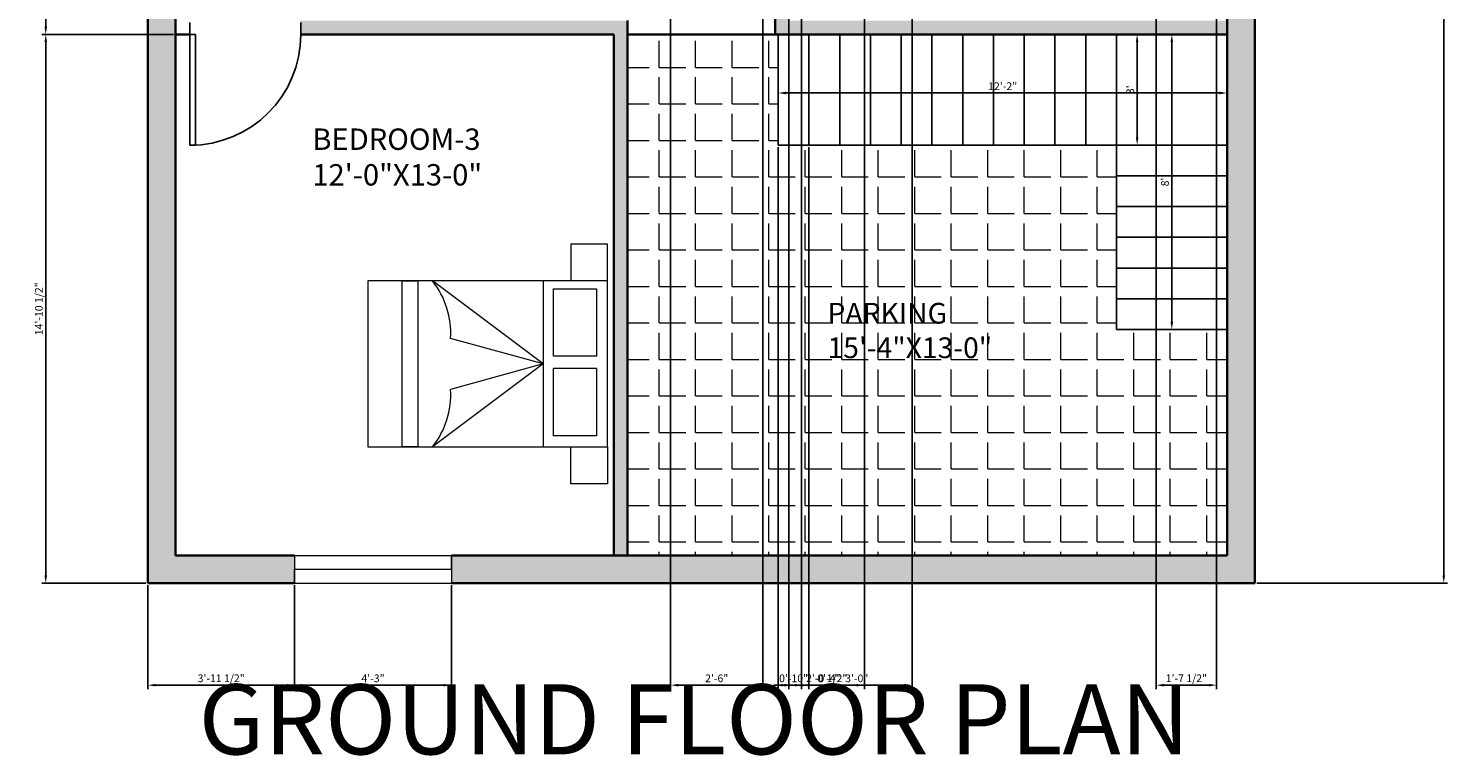
# Model space of a CAD drawing. Units: inches. Extents: x 2063 to 2524, y 2436 to 3097.
# Tile 1 of 4: x 2063 to 2524, y 2436 to 2673. Entities that reach past the tile are written whole.
import ezdxf

# ---------------------------------------------------------------- set-up
doc = ezdxf.new("R2010")
doc.units = ezdxf.units.IN
for name, color, linetype, lineweight in [('A-ANNO-DIMS', 2, 'Continuous', 18), ('A-ANNO-TEXT', 7, 'Continuous', 25), ('A-AREA-IDEN', 7, 'Continuous', 18), ('A-DOOR', 4, 'Continuous', 25), ('A-FLOR-STRS', 7, 'Continuous', 25), ('A-FURN', 8, 'Continuous', 18), ('A-GLAZ', 5, 'Continuous', 18), ('A-WALL', 7, 'Continuous', 35)]:
    doc.layers.add(name, color=color, linetype=linetype, lineweight=lineweight)
doc.layers.add('A-FLOR-PATT', color=252, linetype='Continuous', lineweight=13, true_color=0x939598)
doc.layers.add('A-WALL-PATT', color=251, linetype='Continuous', lineweight=13, true_color=0x636466)
doc.styles.get("Standard").update_dxf_attribs({"font": 'arial.ttf'})
doc.dimstyles.new('ISO-25', dxfattribs={"dimtxt": 2.5, "dimasz": 2.5, "dimexe": 1.25, "dimexo": 0.625, "dimtad": 1, "dimlunit": 3, "dimtxsty": 'Standard', "dimcen": 2.5, "dimadec": 0, "dimazin": 0, "dimtfac": 1, "dimtmove": 0, "dimatfit": 3, "dimfxl": 1, "dimarcsym": 0})

# ---------------------------------------------------------------- blocks, each defined once
blk = doc.blocks.new('*U7')
for p, q in [((0, 0), (0, 4)), ((36, 0), (36, 4))]:
    blk.add_line(p, q)
blk.add_lwpolyline([(0, 0), (0, -36), (1.75, -36), (1.75, 0)], close=True)
blk.add_arc((0, 0), 36, 270, 0)
blk = doc.blocks.new('*D8')
at = {"layer": 'A-ANNO-DIMS', "color": 0, "lineweight": -2, "transparency": 16777216}
for p, q in [((2306.76, 2669.99), (2306.76, 2650.32)), ((2452.76, 2669.99), (2452.76, 2650.32)), ((2450.26, 2651.57), (2309.26, 2651.57))]:
    blk.add_line(p, q, dxfattribs=at)
at = {"layer": 'A-ANNO-DIMS', "color": 0, "transparency": 16777216}
for points in [[(2309.26, 2651.99), (2309.26, 2651.15), (2306.76, 2651.57)], [(2450.26, 2651.99), (2450.26, 2651.15), (2452.76, 2651.57)]]:
    blk.add_solid(points, dxfattribs=at)
at = {"layer": 'Defpoints', "color": 0, "transparency": 16777216}
for p in [(2306.76, 2670.62), (2452.76, 2670.62), (2306.76, 2651.57)]:
    blk.add_point(p, dxfattribs=at)
at = {"layer": 'A-ANNO-DIMS', "color": 0, "transparency": 16777216, "insert": (2379.76, 2653.45), "char_height": 2.5, "attachment_point": 5}
blk.add_mtext('12\'-2"', dxfattribs=at)
blk = doc.blocks.new('*D9')
at = {"layer": 'A-ANNO-DIMS', "color": 0, "lineweight": -2, "transparency": 16777216}
for p, q in [((2452.14, 2670.62), (2433.51, 2670.62)), ((2434.76, 2668.12), (2434.76, 2577.12)), ((2452.14, 2574.62), (2433.51, 2574.62))]:
    blk.add_line(p, q, dxfattribs=at)
at = {"layer": 'A-ANNO-DIMS', "color": 0, "transparency": 16777216}
for points in [[(2434.35, 2668.12), (2435.18, 2668.12), (2434.76, 2670.62)], [(2434.35, 2577.12), (2435.18, 2577.12), (2434.76, 2574.62)]]:
    blk.add_solid(points, dxfattribs=at)
at = {"layer": 'Defpoints', "color": 0, "transparency": 16777216}
for p in [(2452.76, 2670.62), (2434.76, 2574.62), (2452.76, 2574.62)]:
    blk.add_point(p, dxfattribs=at)
at = {"layer": 'A-ANNO-DIMS', "color": 0, "transparency": 16777216, "insert": (2432.86, 2622.62), "char_height": 2.5, "attachment_point": 5, "rotation": 90}
blk.add_mtext("8'", dxfattribs=at)
blk = doc.blocks.new('*D10')
at = {"layer": 'A-ANNO-DIMS', "color": 0, "lineweight": -2, "transparency": 16777216}
for p, q in [((2417.39, 2670.62), (2424.73, 2670.62)), ((2423.48, 2668.12), (2423.48, 2637.12)), ((2417.39, 2634.62), (2424.73, 2634.62))]:
    blk.add_line(p, q, dxfattribs=at)
at = {"layer": 'A-ANNO-DIMS', "color": 0, "transparency": 16777216}
for points in [[(2423.07, 2668.12), (2423.9, 2668.12), (2423.48, 2670.62)], [(2423.07, 2637.12), (2423.9, 2637.12), (2423.48, 2634.62)]]:
    blk.add_solid(points, dxfattribs=at)
at = {"layer": 'Defpoints', "color": 0, "transparency": 16777216}
for p in [(2416.76, 2670.62), (2416.76, 2634.62), (2423.48, 2634.62)]:
    blk.add_point(p, dxfattribs=at)
at = {"layer": 'A-ANNO-DIMS', "color": 0, "transparency": 16777216, "insert": (2421.58, 2652.62), "char_height": 2.5, "attachment_point": 5, "rotation": 90}
blk.add_mtext("3'", dxfattribs=at)
blk = doc.blocks.new('*D15')
at = {"layer": 'A-ANNO-DIMS', "color": 0, "lineweight": -2, "transparency": 16777216}
for p, q in [((2462.39, 3056.12), (2524.46, 3056.12)), ((2523.21, 3053.62), (2523.21, 2494.62)), ((2462.39, 2492.12), (2524.46, 2492.12))]:
    blk.add_line(p, q, dxfattribs=at)
at = {"layer": 'A-ANNO-DIMS', "color": 0, "transparency": 16777216}
for points in [[(2522.79, 3053.62), (2523.62, 3053.62), (2523.21, 3056.12)], [(2522.79, 2494.62), (2523.62, 2494.62), (2523.21, 2492.12)]]:
    blk.add_solid(points, dxfattribs=at)
at = {"layer": 'Defpoints', "color": 0, "transparency": 16777216}
for p in [(2461.76, 3056.12), (2461.76, 2492.12), (2523.21, 2492.12)]:
    blk.add_point(p, dxfattribs=at)
at = {"layer": 'A-ANNO-DIMS', "color": 0, "transparency": 16777216, "insert": (2521.33, 2774.12), "char_height": 2.5, "attachment_point": 5, "rotation": 90}
blk.add_mtext("47'", dxfattribs=at)
blk = doc.blocks.new('BED-DOUBLE-WITH-NIGHTSTANDS')
for p, q in [((12, 78), (0, 78)), ((0, 78), (0, 66)), ((36.48, 74.39), (36.48, 60.42)), ((40.48, 74.39), (40.48, 60.42)), ((66, 78), (78, 78)), ((78, 78), (78, 66)), ((0, 66), (12, 66)), ((77, 66), (66, 66)), ((78, 66), (77, 66)), ((12, 57.08), (66, 57.08)), ((39, 57.08), (12, 21.08)), ((39, 57.08), (30.7, 26.92)), ((39, 57.08), (66, 21.08)), ((39, 57.08), (47.3, 26.92))]:
    blk.add_line(p, q)
for points in [[(12, 0), (66, 0), (66, 78), (12, 78)], [(12, 16.31), (66, 16.31), (66, 11.16), (12, 11.16)]]:
    blk.add_lwpolyline(points, close=True)
for points in [[(36.48, 60.42), (14.53, 60.42), (14.53, 74.39), (36.48, 74.39)], [(40.48, 74.39), (62.43, 74.39), (62.43, 60.42), (40.48, 60.42)]]:
    blk.add_lwpolyline(points)
for centre, start, end in [((29, -0.5), 86.4578, 128.2353), ((49, -0.5), 51.7647, 93.5422)]:
    blk.add_arc(centre, 27.47, start, end)
blk = doc.blocks.new('*D28')
at = {"layer": 'A-ANNO-DIMS', "color": 0, "lineweight": -2, "transparency": 16777216}
for p, q in [((2101.76, 2491.49), (2101.76, 2457.67)), ((2149.48, 2491.49), (2149.48, 2457.67)), ((2104.26, 2458.92), (2146.98, 2458.92))]:
    blk.add_line(p, q, dxfattribs=at)
at = {"layer": 'A-ANNO-DIMS', "color": 0, "transparency": 16777216}
for points in [[(2104.26, 2459.33), (2104.26, 2458.5), (2101.76, 2458.92)], [(2146.98, 2459.33), (2146.98, 2458.5), (2149.48, 2458.92)]]:
    blk.add_solid(points, dxfattribs=at)
at = {"layer": 'Defpoints', "color": 0, "transparency": 16777216}
for p in [(2101.76, 2492.12), (2149.48, 2492.12), (2149.48, 2458.92)]:
    blk.add_point(p, dxfattribs=at)
at = {"layer": 'A-ANNO-DIMS', "color": 0, "transparency": 16777216, "insert": (2125.62, 2460.84), "char_height": 2.5, "attachment_point": 5}
blk.add_mtext('3\'-11 1/2"', dxfattribs=at)
blk = doc.blocks.new('*D29')
at = {"layer": 'A-ANNO-DIMS', "color": 0, "lineweight": -2, "transparency": 16777216}
for p, q in [((2149.48, 2491.49), (2149.48, 2457.67)), ((2200.48, 2491.49), (2200.48, 2457.67)), ((2151.98, 2458.92), (2197.98, 2458.92))]:
    blk.add_line(p, q, dxfattribs=at)
at = {"layer": 'A-ANNO-DIMS', "color": 0, "transparency": 16777216}
for points in [[(2151.98, 2459.33), (2151.98, 2458.5), (2149.48, 2458.92)], [(2197.98, 2459.33), (2197.98, 2458.5), (2200.48, 2458.92)]]:
    blk.add_solid(points, dxfattribs=at)
at = {"layer": 'Defpoints', "color": 0, "transparency": 16777216}
for p in [(2149.48, 2492.12), (2200.48, 2492.12), (2200.48, 2458.92)]:
    blk.add_point(p, dxfattribs=at)
at = {"layer": 'A-ANNO-DIMS', "color": 0, "transparency": 16777216, "insert": (2174.98, 2460.82), "char_height": 2.5, "attachment_point": 5}
blk.add_mtext('4\'-3"', dxfattribs=at)
blk = doc.blocks.new('*D30')
at = {"layer": 'A-ANNO-DIMS', "color": 0, "lineweight": -2, "transparency": 16777216}
for p, q in [((2110.14, 2670.62), (2067.31, 2670.62)), ((2068.56, 2494.62), (2068.56, 2668.12)), ((2101.14, 2492.12), (2067.31, 2492.12))]:
    blk.add_line(p, q, dxfattribs=at)
at = {"layer": 'A-ANNO-DIMS', "color": 0, "transparency": 16777216}
for points in [[(2068.15, 2668.12), (2068.98, 2668.12), (2068.56, 2670.62)], [(2068.15, 2494.62), (2068.98, 2494.62), (2068.56, 2492.12)]]:
    blk.add_solid(points, dxfattribs=at)
at = {"layer": 'Defpoints', "color": 0, "transparency": 16777216}
for p in [(2068.56, 2670.62), (2110.76, 2670.62), (2101.76, 2492.12)]:
    blk.add_point(p, dxfattribs=at)
at = {"layer": 'A-ANNO-DIMS', "color": 0, "transparency": 16777216, "insert": (2066.65, 2581.37), "char_height": 2.5, "attachment_point": 5, "rotation": 90}
blk.add_mtext('14\'-10 1/2"', dxfattribs=at)
blk = doc.blocks.new('*D31')
at = {"layer": 'A-ANNO-DIMS', "color": 0, "lineweight": -2, "transparency": 16777216}
for p, q in [((2110.14, 2903.12), (2067.31, 2903.12)), ((2068.56, 2673.12), (2068.56, 2900.62)), ((2110.14, 2670.62), (2067.31, 2670.62))]:
    blk.add_line(p, q, dxfattribs=at)
at = {"layer": 'A-ANNO-DIMS', "color": 0, "transparency": 16777216}
for points in [[(2068.15, 2900.62), (2068.98, 2900.62), (2068.56, 2903.12)], [(2068.15, 2673.12), (2068.98, 2673.12), (2068.56, 2670.62)]]:
    blk.add_solid(points, dxfattribs=at)
at = {"layer": 'Defpoints', "color": 0, "transparency": 16777216}
for p in [(2068.56, 2903.12), (2110.76, 2903.12), (2110.76, 2670.62)]:
    blk.add_point(p, dxfattribs=at)
at = {"layer": 'A-ANNO-DIMS', "color": 0, "transparency": 16777216, "insert": (2066.65, 2786.87), "char_height": 2.5, "attachment_point": 5, "rotation": 90}
blk.add_mtext('19\'-4 1/2"', dxfattribs=at)
blk = doc.blocks.new('*D34')
at = {"layer": 'A-ANNO-DIMS', "color": 0, "lineweight": -2, "transparency": 16777216}
for p, q in [((2271.76, 2914.94), (2271.76, 2457.67)), ((2301.76, 2914.94), (2301.76, 2457.67)), ((2274.26, 2458.92), (2299.26, 2458.92))]:
    blk.add_line(p, q, dxfattribs=at)
at = {"layer": 'A-ANNO-DIMS', "color": 0, "transparency": 16777216}
for points in [[(2274.26, 2459.33), (2274.26, 2458.5), (2271.76, 2458.92)], [(2299.26, 2459.33), (2299.26, 2458.5), (2301.76, 2458.92)]]:
    blk.add_solid(points, dxfattribs=at)
at = {"layer": 'Defpoints', "color": 0, "transparency": 16777216}
for p in [(2271.76, 2915.57), (2301.76, 2915.57), (2301.76, 2458.92)]:
    blk.add_point(p, dxfattribs=at)
at = {"layer": 'A-ANNO-DIMS', "color": 0, "transparency": 16777216, "insert": (2286.76, 2460.82), "char_height": 2.5, "attachment_point": 5}
blk.add_mtext('2\'-6"', dxfattribs=at)
blk = doc.blocks.new('*D36')
at = {"layer": 'A-ANNO-DIMS', "color": 0, "lineweight": -2, "transparency": 16777216}
for p, q in [((2314.3, 2902.49), (2314.3, 2457.67)), ((2350.3, 2902.49), (2350.3, 2457.67)), ((2316.8, 2458.92), (2347.8, 2458.92))]:
    blk.add_line(p, q, dxfattribs=at)
at = {"layer": 'A-ANNO-DIMS', "color": 0, "transparency": 16777216}
for points in [[(2316.8, 2459.33), (2316.8, 2458.5), (2314.3, 2458.92)], [(2347.8, 2459.33), (2347.8, 2458.5), (2350.3, 2458.92)]]:
    blk.add_solid(points, dxfattribs=at)
at = {"layer": 'Defpoints', "color": 0, "transparency": 16777216}
for p in [(2314.3, 2903.12), (2350.3, 2903.12), (2350.3, 2458.92)]:
    blk.add_point(p, dxfattribs=at)
at = {"layer": 'A-ANNO-DIMS', "color": 0, "transparency": 16777216, "insert": (2332.3, 2460.82), "char_height": 2.5, "attachment_point": 5}
blk.add_mtext('3\'-0"', dxfattribs=at)
blk = doc.blocks.new('*D43')
at = {"layer": 'A-ANNO-DIMS', "color": 0, "lineweight": -2, "transparency": 16777216}
for p, q in [((2429.67, 2709.7), (2429.67, 2457.67)), ((2449.35, 2709.7), (2449.35, 2457.67)), ((2432.17, 2458.92), (2446.85, 2458.92))]:
    blk.add_line(p, q, dxfattribs=at)
at = {"layer": 'A-ANNO-DIMS', "color": 0, "transparency": 16777216}
for points in [[(2432.17, 2459.33), (2432.17, 2458.5), (2429.67, 2458.92)], [(2446.85, 2459.33), (2446.85, 2458.5), (2449.35, 2458.92)]]:
    blk.add_solid(points, dxfattribs=at)
at = {"layer": 'Defpoints', "color": 0, "transparency": 16777216}
for p in [(2429.67, 2710.33), (2449.35, 2710.33), (2449.35, 2458.92)]:
    blk.add_point(p, dxfattribs=at)
at = {"layer": 'A-ANNO-DIMS', "color": 0, "transparency": 16777216, "insert": (2439.51, 2460.84), "char_height": 2.5, "attachment_point": 5}
blk.add_mtext('1\'-7 1/2"', dxfattribs=at)
blk = doc.blocks.new('*D46')
at = {"layer": 'A-ANNO-DIMS', "color": 0, "lineweight": -2, "transparency": 16777216}
for p, q in [((2306.76, 2633.99), (2306.76, 2457.67)), ((2316.76, 2633.99), (2316.76, 2457.67)), ((2309.26, 2458.92), (2314.26, 2458.92))]:
    blk.add_line(p, q, dxfattribs=at)
at = {"layer": 'A-ANNO-DIMS', "color": 0, "transparency": 16777216}
for points in [[(2309.26, 2459.33), (2309.26, 2458.5), (2306.76, 2458.92)], [(2314.26, 2459.33), (2314.26, 2458.5), (2316.76, 2458.92)]]:
    blk.add_solid(points, dxfattribs=at)
at = {"layer": 'Defpoints', "color": 0, "transparency": 16777216}
for p in [(2306.76, 2634.62), (2316.76, 2634.62), (2316.76, 2458.92)]:
    blk.add_point(p, dxfattribs=at)
at = {"layer": 'A-ANNO-DIMS', "color": 0, "transparency": 16777216, "insert": (2311.76, 2460.82), "char_height": 2.5, "attachment_point": 5}
blk.add_mtext('0\'-10"', dxfattribs=at)
blk = doc.blocks.new('*D48')
at = {"layer": 'A-ANNO-DIMS', "color": 0, "lineweight": -2, "transparency": 16777216}
for p, q in [((2310.26, 2906.99), (2310.26, 2457.67)), ((2314.3, 2902.49), (2314.3, 2457.67)), ((2307.76, 2458.92), (2305.26, 2458.92)), ((2310.26, 2458.92), (2314.3, 2458.92)), ((2316.8, 2458.92), (2327.2, 2458.92))]:
    blk.add_line(p, q, dxfattribs=at)
at = {"layer": 'A-ANNO-DIMS', "color": 0, "transparency": 16777216}
for points in [[(2307.76, 2459.33), (2307.76, 2458.5), (2310.26, 2458.92)], [(2316.8, 2459.33), (2316.8, 2458.5), (2314.3, 2458.92)]]:
    blk.add_solid(points, dxfattribs=at)
at = {"layer": 'Defpoints', "color": 0, "transparency": 16777216}
for p in [(2310.26, 2907.62), (2314.3, 2903.12), (2314.3, 2458.92)]:
    blk.add_point(p, dxfattribs=at)
at = {"layer": 'A-ANNO-DIMS', "color": 0, "transparency": 16777216, "insert": (2323.25, 2460.82), "char_height": 2.5, "attachment_point": 5}
blk.add_mtext('0\'-4"', dxfattribs=at)
blk = doc.blocks.new('*D51')
at = {"layer": 'A-ANNO-DIMS', "color": 0, "lineweight": -2, "transparency": 16777216}
for p, q in [((2310.26, 2674.49), (2310.26, 2457.67)), ((2334.8, 2676.36), (2334.8, 2457.67)), ((2312.76, 2458.92), (2332.3, 2458.92))]:
    blk.add_line(p, q, dxfattribs=at)
at = {"layer": 'A-ANNO-DIMS', "color": 0, "transparency": 16777216}
for points in [[(2312.76, 2459.33), (2312.76, 2458.5), (2310.26, 2458.92)], [(2332.3, 2459.33), (2332.3, 2458.5), (2334.8, 2458.92)]]:
    blk.add_solid(points, dxfattribs=at)
at = {"layer": 'Defpoints', "color": 0, "transparency": 16777216}
for p in [(2334.8, 2676.99), (2310.26, 2675.12), (2334.8, 2458.92)]:
    blk.add_point(p, dxfattribs=at)
at = {"layer": 'A-ANNO-DIMS', "color": 0, "transparency": 16777216, "insert": (2322.53, 2460.84), "char_height": 2.5, "attachment_point": 5}
blk.add_mtext('2\'-0 1/2"', dxfattribs=at)

msp = doc.modelspace()

# ---------------------------------------------------------------- hatches: boundary and pattern name
at = {"layer": 'A-FLOR-PATT'}
h = msp.add_hatch(dxfattribs=at)
h.set_pattern_fill('ANGLE', color=256, scale=1.7)
h.set_pattern_definition([(0, (0, 0), (0, 11.8745), [8.636, -3.2385]), (90, (0, 0), (-11.8745, 7e-16), [8.636, -3.2385])])
h.paths.add_polyline_path([(2416.763, 2634.618), (2316.763, 2634.618), (2306.763, 2634.618), (2306.763, 2670.618), (2305.763, 2670.618), (2257.763, 2670.618), (2257.763, 2501.118), (2452.763, 2501.118), (2452.763, 2574.618), (2416.763, 2574.618), (2416.763, 2584.618)])
at = {"layer": 'A-WALL-PATT'}
h = msp.add_hatch(color=256, dxfattribs=at)
h.dxf.hatch_style = 1
h.paths.add_polyline_path([(2110.763, 2670.618), (2110.763, 2676.643), (2110.763, 3047.118), (2452.763, 3047.118), (2452.763, 2501.118), (2200.478, 2501.118), (2200.478, 2492.118), (2461.763, 2492.118), (2461.763, 3056.118), (2101.763, 3056.118), (2101.763, 2492.118), (2149.478, 2492.118), (2149.478, 2496.618), (2149.478, 2501.118), (2110.763, 2501.118)])
h.paths.add_polyline_path([(2257.763, 2675.118), (2257.255, 2675.091), (2253.255, 2675.091), (2213.255, 2675.091), (2151.474, 2675.107), (2151.474, 2674.543), (2151.474, 2670.618), (2253.263, 2670.618), (2253.263, 2501.118), (2257.763, 2501.118)], flags=17)
h.paths.add_polyline_path([(2310.263, 3006.972), (2305.763, 3006.972), (2305.763, 2920.067), (2301.763, 2920.067), (2301.759, 2920.067), (2301.759, 2920.063), (2301.759, 2916.063), (2301.759, 2915.567), (2305.763, 2915.567), (2305.763, 2903.118), (2314.3, 2903.118), (2314.3, 2903.618), (2314.3, 2907.618), (2310.263, 2907.618)], flags=17)
h.paths.add_polyline_path([(2257.763, 3006.972), (2253.263, 3006.972), (2253.263, 2907.618), (2249.263, 2907.618), (2249.258, 2907.618), (2249.258, 2907.597), (2249.258, 2903.597), (2249.258, 2903.118), (2257.763, 2903.118), (2257.763, 2915.567), (2271.759, 2915.567), (2271.759, 2916.063), (2271.759, 2920.067), (2257.763, 2920.067)], flags=17)
h.paths.add_polyline_path([(2213.258, 2907.618), (2110.763, 2907.618), (2110.763, 2903.118), (2213.258, 2903.118), (2213.258, 2903.597)], flags=17)
h.paths.add_polyline_path([(2411.763, 2907.618), (2350.3, 2907.618), (2350.3, 2903.618), (2350.3, 2903.118), (2407.264, 2903.118), (2411.763, 2903.118)], flags=17)
h.paths.add_polyline_path([(2260.327, 2964.034), (2307.905, 2964.034), (2307.905, 2989.359), (2260.327, 2989.359)], flags=25)
h = msp.add_hatch(color=256, dxfattribs=at)
h.dxf.hatch_style = 1
h.paths.add_polyline_path([(2310.263, 2811.618), (2305.763, 2811.618), (2253.263, 2811.618), (2253.263, 2716.118), (2253.255, 2715.091), (2257.255, 2715.091), (2257.763, 2715.091), (2257.763, 2720.618), (2257.763, 2807.118), (2305.763, 2807.118), (2305.763, 2799.95), (2305.776, 2799.95), (2309.776, 2799.95), (2310.263, 2799.95)])
h.paths.add_polyline_path([(2310.263, 2769.95), (2309.776, 2769.95), (2305.763, 2769.95), (2305.763, 2720.618), (2257.763, 2720.618), (2257.763, 2716.118), (2305.763, 2716.118), (2305.763, 2670.618), (2310.263, 2670.618), (2452.763, 2670.618), (2452.763, 2675.118), (2426.899, 2675.118), (2310.263, 2675.118)])

# ---------------------------------------------------------------- linework, layer by layer
at = {"layer": 'A-FLOR-STRS'}
for p, q in [((2306.763, 2670.618), (2306.763, 2634.618)), ((2306.763, 2670.618), (2306.763, 2634.618)), ((2316.763, 2634.618), (2316.763, 2670.618)), ((2326.763, 2634.618), (2326.763, 2670.618)), ((2336.763, 2634.618), (2336.763, 2670.618)), ((2346.763, 2634.618), (2346.763, 2670.618)), ((2356.763, 2634.618), (2356.763, 2670.618)), ((2366.763, 2634.618), (2366.763, 2670.618)), ((2376.763, 2634.618), (2376.763, 2670.618)), ((2386.763, 2634.618), (2386.763, 2670.618)), ((2396.763, 2634.618), (2396.763, 2670.618)), ((2406.763, 2634.618), (2406.763, 2670.618)), ((2416.763, 2634.618), (2416.763, 2670.618)), ((2306.763, 2634.618), (2316.763, 2634.618)), ((2316.763, 2634.618), (2416.763, 2634.618)), ((2416.763, 2634.618), (2452.763, 2634.618)), ((2416.763, 2634.618), (2416.763, 2584.618)), ((2416.763, 2624.618), (2452.763, 2624.618)), ((2416.763, 2614.618), (2452.763, 2614.618)), ((2416.763, 2604.618), (2452.763, 2604.618)), ((2416.763, 2594.618), (2452.763, 2594.618)), ((2416.763, 2594.618), (2452.763, 2594.618)), ((2416.763, 2584.618), (2452.763, 2584.618)), ((2416.763, 2584.618), (2416.763, 2574.618)), ((2416.763, 2574.618), (2452.763, 2574.618))]:
    msp.add_line(p, q, dxfattribs=at)
at = {"layer": 'A-GLAZ'}
for p, q in [((2149.478, 2501.118), (2149.478, 2492.118)), ((2149.478, 2501.118), (2200.478, 2501.118)), ((2200.478, 2496.618), (2200.478, 2501.118)), ((2200.478, 2501.118), (2200.478, 2492.118)), ((2149.478, 2492.118), (2149.478, 2496.618)), ((2149.478, 2496.618), (2200.478, 2496.618)), ((2149.478, 2492.118), (2200.478, 2492.118))]:
    msp.add_line(p, q, dxfattribs=at)
at = {"layer": 'A-WALL'}
for p, q in [((2101.763, 2492.118), (2101.763, 3056.118)), ((2461.763, 3056.118), (2461.763, 2492.118)), ((2452.763, 3047.118), (2452.763, 2501.118)), ((2305.763, 2716.118), (2305.763, 2670.618)), ((2110.763, 2670.618), (2110.763, 2676.643)), ((2257.763, 2501.118), (2257.763, 2675.118)), ((2110.763, 2501.118), (2110.763, 2670.618)), ((2115.474, 2670.618), (2110.763, 2670.618)), ((2253.263, 2670.618), (2151.474, 2670.618)), ((2253.263, 2501.118), (2253.263, 2670.618)), ((2305.763, 2670.618), (2257.763, 2670.618)), ((2305.763, 2670.618), (2310.263, 2670.618)), ((2452.763, 2670.618), (2306.763, 2670.618)), ((2452.763, 2670.618), (2310.263, 2670.618)), ((2149.478, 2501.118), (2110.763, 2501.118)), ((2452.763, 2501.118), (2200.478, 2501.118)), ((2149.478, 2492.118), (2101.763, 2492.118)), ((2461.763, 2492.118), (2200.478, 2492.118))]:
    msp.add_line(p, q, dxfattribs=at)

# ---------------------------------------------------------------- block references
at = {"layer": 'A-DOOR'}
msp.add_blockref('*U7', (2115.474, 2670.543), dxfattribs=at)
at = {"layer": 'A-FURN', "rotation": 269.9999999999978}
msp.add_blockref('BED-DOUBLE-WITH-NIGHTSTANDS', (2173.29, 2602.422), dxfattribs=at)

# ---------------------------------------------------------------- texts
at = {"layer": 'A-ANNO-TEXT', "insert": (2118.282, 2459.198), "char_height": 22.79082, "attachment_point": 1}
msp.add_mtext_dynamic_manual_height_columns('GROUND FLOOR PLAN', width=3477.15223, gutter_width=113.954, heights=[2.91], dxfattribs=at)
at = {"layer": 'A-AREA-IDEN', "attachment_point": 1}
for s, width, gutter_width, insert, char_height in [('BEDROOM-3\\P12\'-0"X13-0"', 138.69556, 34.769, (2155.254, 2640.01), 6.95382), ('PARKING\\P15\'-4"X13-0"', 132.76108, 33.695, (2322.808, 2583.285), 6.73894)]:
    msp.add_mtext_dynamic_manual_height_columns(s, width=width, gutter_width=gutter_width, heights=[0], dxfattribs=dict(at, insert=insert, char_height=char_height))

# ---------------------------------------------------------------- dimensions: what is measured, and where the dimension line sits
at = {"layer": 'A-ANNO-DIMS'}
for base, p1, p2, override, picture, middle in [((2523.206, 2492.118), (2461.763, 3056.118), (2461.763, 2492.118), {"dimclrd": 0, "dimclre": 0, "dimclrt": 0}, '*D15', (2521.331, 2774.118)), ((2068.563, 2903.118), (2110.763, 2670.618), (2110.763, 2903.118), {"dimdec": 1, "dimlfac": 1, "dimrnd": 0, "dimzin": 1, "dimdsep": 46, "dimlunit": 4, "dimfrac": 2}, '*D31', (2066.646, 2786.868)), ((2068.563, 2670.618), (2101.763, 2492.118), (2110.763, 2670.618), {"dimdec": 1, "dimlfac": 1, "dimrnd": 0, "dimzin": 1, "dimdsep": 46, "dimlunit": 4, "dimfrac": 2}, '*D30', (2066.646, 2581.368)), ((2423.485, 2634.618), (2416.763, 2670.618), (2416.763, 2634.618), {"dimclrd": 0, "dimclre": 0, "dimclrt": 0}, '*D10', (2421.583, 2652.618)), ((2434.763, 2574.618), (2452.763, 2670.618), (2452.763, 2574.618), {"dimclrd": 0, "dimclre": 0, "dimclrt": 0}, '*D9', (2432.862, 2622.618))]:
    dim = msp.add_linear_dim(base=base, p1=p1, p2=p2, angle=90, dimstyle='ISO-25', override=override, dxfattribs=at)
    dim.commit()
    dim.dimension.update_dxf_attribs({"geometry": picture, "text_midpoint": middle})
for base, p1, p2, override, picture, middle in [((2301.759, 2458.918), (2271.759, 2915.567), (2301.759, 2915.567), {"dimdec": 1, "dimlfac": 1, "dimrnd": 0, "dimzin": 1, "dimdsep": 46, "dimlunit": 4, "dimfrac": 2}, '*D34', (2286.759, 2460.819)), ((2314.3, 2458.918), (2310.263, 2907.618), (2314.3, 2903.118), {"dimdec": 1, "dimlfac": 1, "dimrnd": 0, "dimzin": 1, "dimdsep": 46, "dimlunit": 4, "dimfrac": 2}, '*D48', (2323.248, 2460.819)), ((2350.3, 2458.918), (2314.3, 2903.118), (2350.3, 2903.118), {"dimdec": 1, "dimlfac": 1, "dimrnd": 0, "dimzin": 1, "dimdsep": 46, "dimlunit": 4, "dimfrac": 2}, '*D36', (2332.3, 2460.82)), ((2449.352, 2458.918), (2429.674, 2710.326), (2449.352, 2710.326), {"dimdec": 1, "dimlfac": 1, "dimrnd": 0, "dimzin": 1, "dimdsep": 46, "dimlunit": 4, "dimfrac": 2}, '*D43', (2439.513, 2460.835)), ((2334.798, 2458.918), (2310.263, 2675.118), (2334.798, 2676.988), {"dimdec": 1, "dimlfac": 1, "dimrnd": 0, "dimzin": 1, "dimdsep": 46, "dimlunit": 4, "dimfrac": 2}, '*D51', (2322.531, 2460.835)), ((2306.763, 2651.569), (2452.763, 2670.618), (2306.763, 2670.618), {"dimclrd": 0, "dimclre": 0, "dimclrt": 0}, '*D8', (2379.763, 2653.449)), ((2316.763, 2458.918), (2306.763, 2634.618), (2316.763, 2634.618), {"dimdec": 1, "dimlfac": 1, "dimrnd": 0, "dimzin": 1, "dimdsep": 46, "dimlunit": 4, "dimfrac": 2}, '*D46', (2311.763, 2460.819)), ((2149.478, 2458.918), (2101.763, 2492.118), (2149.478, 2492.118), {"dimdec": 1, "dimlfac": 1, "dimrnd": 0, "dimzin": 1, "dimdsep": 46, "dimlunit": 4, "dimfrac": 2}, '*D28', (2125.621, 2460.836)), ((2200.478, 2458.918), (2149.478, 2492.118), (2200.478, 2492.118), {"dimdec": 1, "dimlfac": 1, "dimrnd": 0, "dimzin": 1, "dimdsep": 46, "dimlunit": 4, "dimfrac": 2}, '*D29', (2174.978, 2460.82))]:
    dim = msp.add_linear_dim(base=base, p1=p1, p2=p2, dimstyle='ISO-25', override=override, dxfattribs=at)
    dim.commit()
    dim.dimension.update_dxf_attribs({"geometry": picture, "text_midpoint": middle})

doc.saveas('drawing.dxf')
